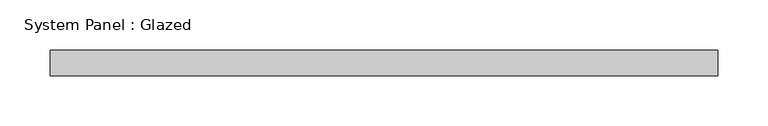
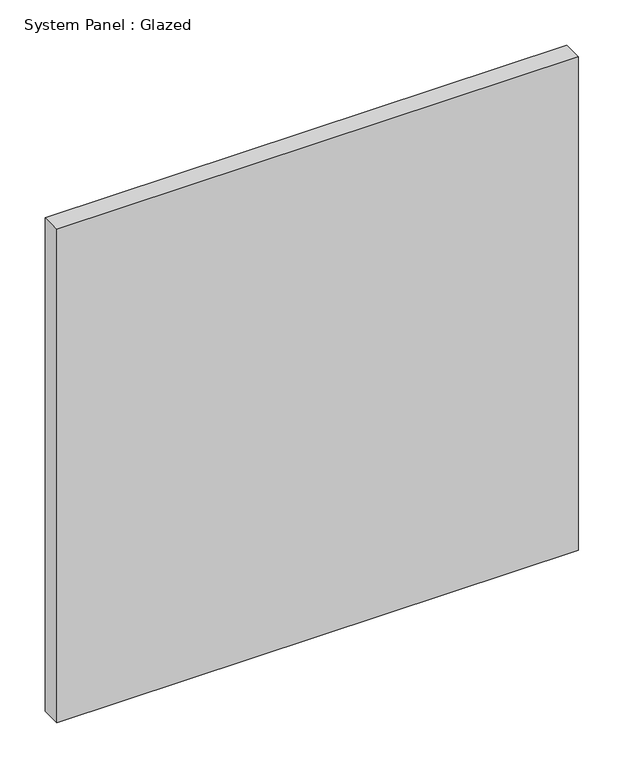
"""IFC4 building model written with IfcOpenShell, lengths in millimetres: plate geometry, System Panel : Glazed."""

from ifc_helpers import new_model, si_unit, origin, origin_with_axes, place, context, project, spatial, polyline, outline, extrude, source, transform, mapped, element, save


def system_panel_glazed_afa25fb8(model_context):
    return source(origin(), model_context, "Body", "SweptSolid", [
        extrude(outline(polyline([(333.375, 19.05), (-333.375, 19.05), (-333.375, 44.45), (333.375, 44.45), (333.375, 19.05)])), origin_with_axes(), (0.0, 0.0, 1.0), 666.75),
    ])


if __name__ == "__main__":
    model = new_model("IFC4")
    model_context = context("Model", 3, world=origin())
    ifc_project = project(units=[si_unit("LENGTHUNIT", "METRE", prefix="MILLI")], contexts=[model_context])
    site = spatial("IfcSite", under=ifc_project)
    building = spatial("IfcBuilding", under=site)
    placement = place(None, origin())
    system_panel_glazed_shape = system_panel_glazed_afa25fb8(model_context)
    element("IfcPlate", 1, ObjectType="System Panel : Glazed", at=placement, inside=building, context=model_context, shape_type="MappedRepresentation", body=[
        mapped(system_panel_glazed_shape, transform((0.0, 0.0, 0.0), x_axis=(1.0, 0.0, 0.0), y_axis=(0.0, 1.0, 0.0), z_axis=(0.0, 0.0, 1.0))),
    ])
    save(model, "model.ifc")

# Revit data of these elements
# Type "System Panel : Glazed"
#   Construction Type Id = "GSP4R"
#   Analytic Construction = "1/8 in Pilkington single glazing"
#   Visual Light Transmittance = 0.9
#   Solar Heat Gain Coefficient = 0.86
#   Heat Transfer Coefficient (U) = 1.18115 BTU/(h·ft²·°F)
# Element 1 (IfcPlate, "System Panel : Glazed")
#   Materials on its faces: "Glass"
# Materials
#   "Glass": class "Glass", colour RGB 0 128 192, transparency 0.75, Description = "Soda Lime Glass", Cost = 0
